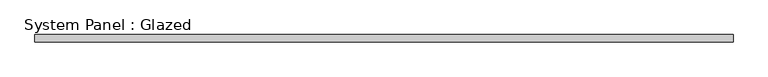
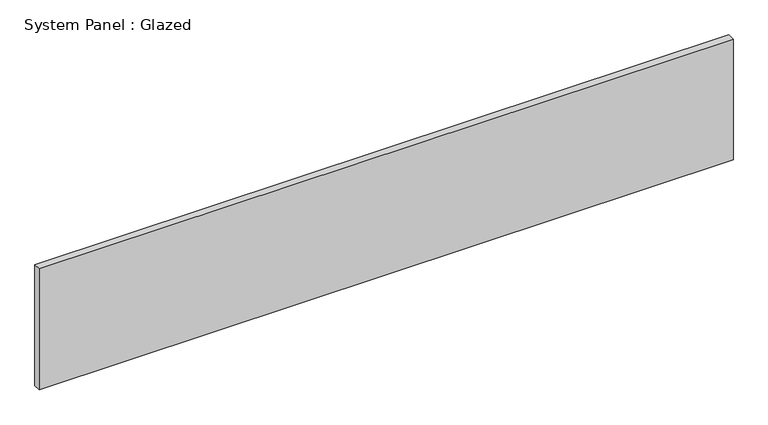
"""IFC4 building model written with IfcOpenShell, lengths in millimetres: plate geometry, System Panel : Glazed."""

from ifc_helpers import new_model, si_unit, origin, origin_with_axes, place, context, project, spatial, polyline, outline, extrude, source, transform, mapped, element, save


def system_panel_glazed_5c06d9ac(model_context):
    return source(origin(), model_context, "Body", "SweptSolid", [
        extrude(outline(polyline([(1222.375, 19.05), (-1222.375, 19.05), (-1222.375, 44.45), (1222.375, 44.45), (1222.375, 19.05)])), origin_with_axes(), (0.0, 0.0, 1.0), 450.1068067),
    ])


if __name__ == "__main__":
    model = new_model("IFC4")
    model_context = context("Model", 3, world=origin())
    ifc_project = project(units=[si_unit("LENGTHUNIT", "METRE", prefix="MILLI")], contexts=[model_context])
    site = spatial("IfcSite", under=ifc_project)
    building = spatial("IfcBuilding", under=site)
    placement = place(None, origin())
    system_panel_glazed_shape = system_panel_glazed_5c06d9ac(model_context)
    element("IfcPlate", 1, ObjectType="System Panel : Glazed", at=placement, inside=building, context=model_context, shape_type="MappedRepresentation", body=[
        mapped(system_panel_glazed_shape, transform((0.0, 0.0, 0.0), x_axis=(1.0, 0.0, 0.0), y_axis=(0.0, 1.0, 0.0), z_axis=(0.0, 0.0, 1.0))),
    ])
    save(model, "model.ifc")

# Revit data of these elements
# Type "System Panel : Glazed"
#   Construction Type Id = "GSP4R"
#   Analytic Construction = "1/8 in Pilkington single glazing"
#   Visual Light Transmittance = 0.9
#   Solar Heat Gain Coefficient = 0.86
#   Heat Transfer Coefficient (U) = 1.18115 BTU/(h·ft²·°F)
#   Define Thermal Properties by = 1
# Element 1 (IfcPlate, "System Panel : Glazed")
#   Materials on its faces: "Glass"
# Materials
#   "Glass": class "Glass", colour RGB 0 128 192, transparency 0.75, Description = "Soda Lime Glass", Cost = 0
